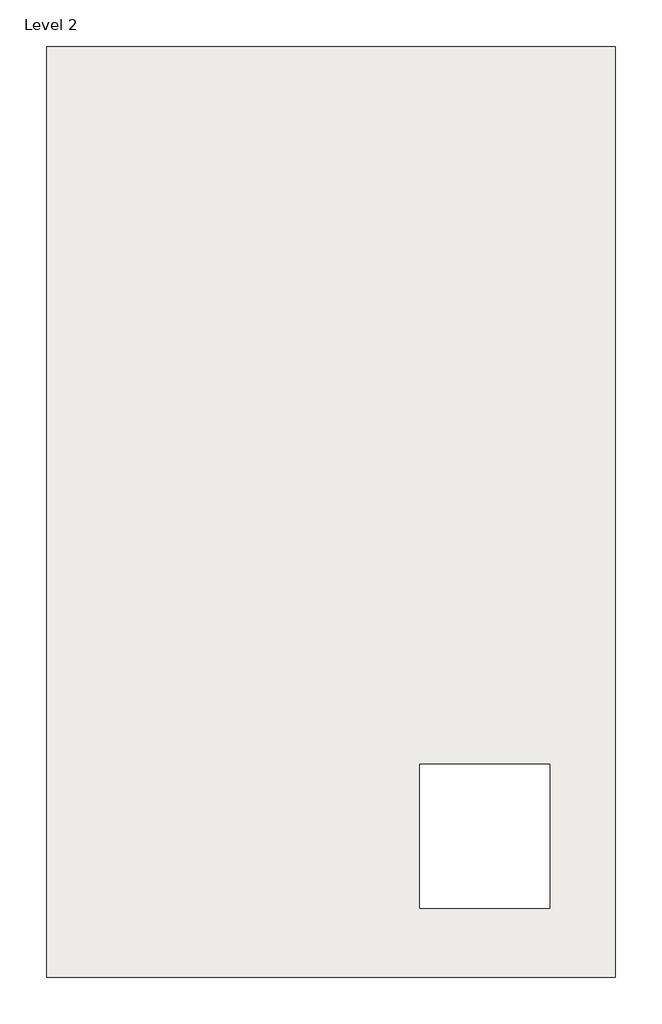
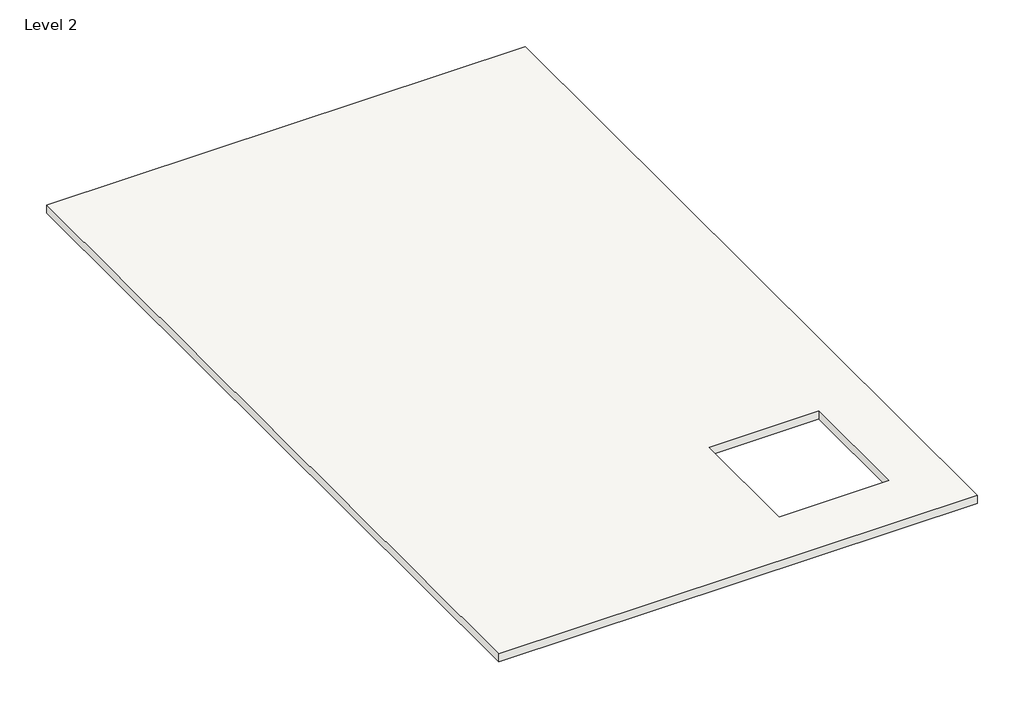
# One storey: 1 roof.
"""IFC4 building model written with IfcOpenShell, lengths in millimetres."""

from ifc_helpers import new_model, si_unit, frame, origin, place, context, project, spatial, polyline, outline, extrude, element, save

model = new_model("IFC4")

# Units and contexts
model_context = context("Model", 3, world=origin())
ifc_project = project(units=[si_unit("LENGTHUNIT", "METRE", prefix="MILLI")], contexts=[model_context])

# Site, building, storey
site = spatial("IfcSite", under=ifc_project)
building = spatial("IfcBuilding", under=site)
storey = spatial("IfcBuildingStorey", under=building, Name="Level 2", Elevation=3048.0)

# Roof
placement = place(None, origin())
element("IfcRoof", 1, ObjectType="Generic - 12\"", at=placement, inside=storey, context=model_context, shape_type="SweptSolid", body=[
    extrude(outline(polyline([(-5503.3915084, -6415.0564015), (-5503.3915084, 7491.4435985), (2992.9084916, 7491.4435985), (2992.9084916, -6415.0564015), (-5503.3915084, -6415.0564015)]), holes=[polyline([(2014.669115, -3231.9425028), (68.5389801, -3231.9425028), (68.5389801, -5380.9250672), (2014.669115, -5380.9250672), (2014.669115, -3231.9425028)])]), frame((0.0, 0.0, 3048.0), z_axis=(0.0, 0.0, 1.0), x_axis=(1.0, 0.0, 0.0)), (0.0, 0.0, 1.0), 152.4),
])

save(model, "model.ifc")

# Revit data of these elements
# Type "Generic - 12\""
#   Assembly Code = "B1020"
#   Layers, outside or top first: 0' - 6" no material (function 1)
# Element 1 (IfcRoof, "Generic - 12\"")
#   built-in parameter 1001705 = 10.5 (stored number, unit not read)
#   built-in parameter 1001710 = 33615
#   Phase Created = New Construction
#   Materials on its faces: "Default Roof"
# Materials
#   "Default Roof": colour RGB 88 101 114, transparency 0, Cost = 0
